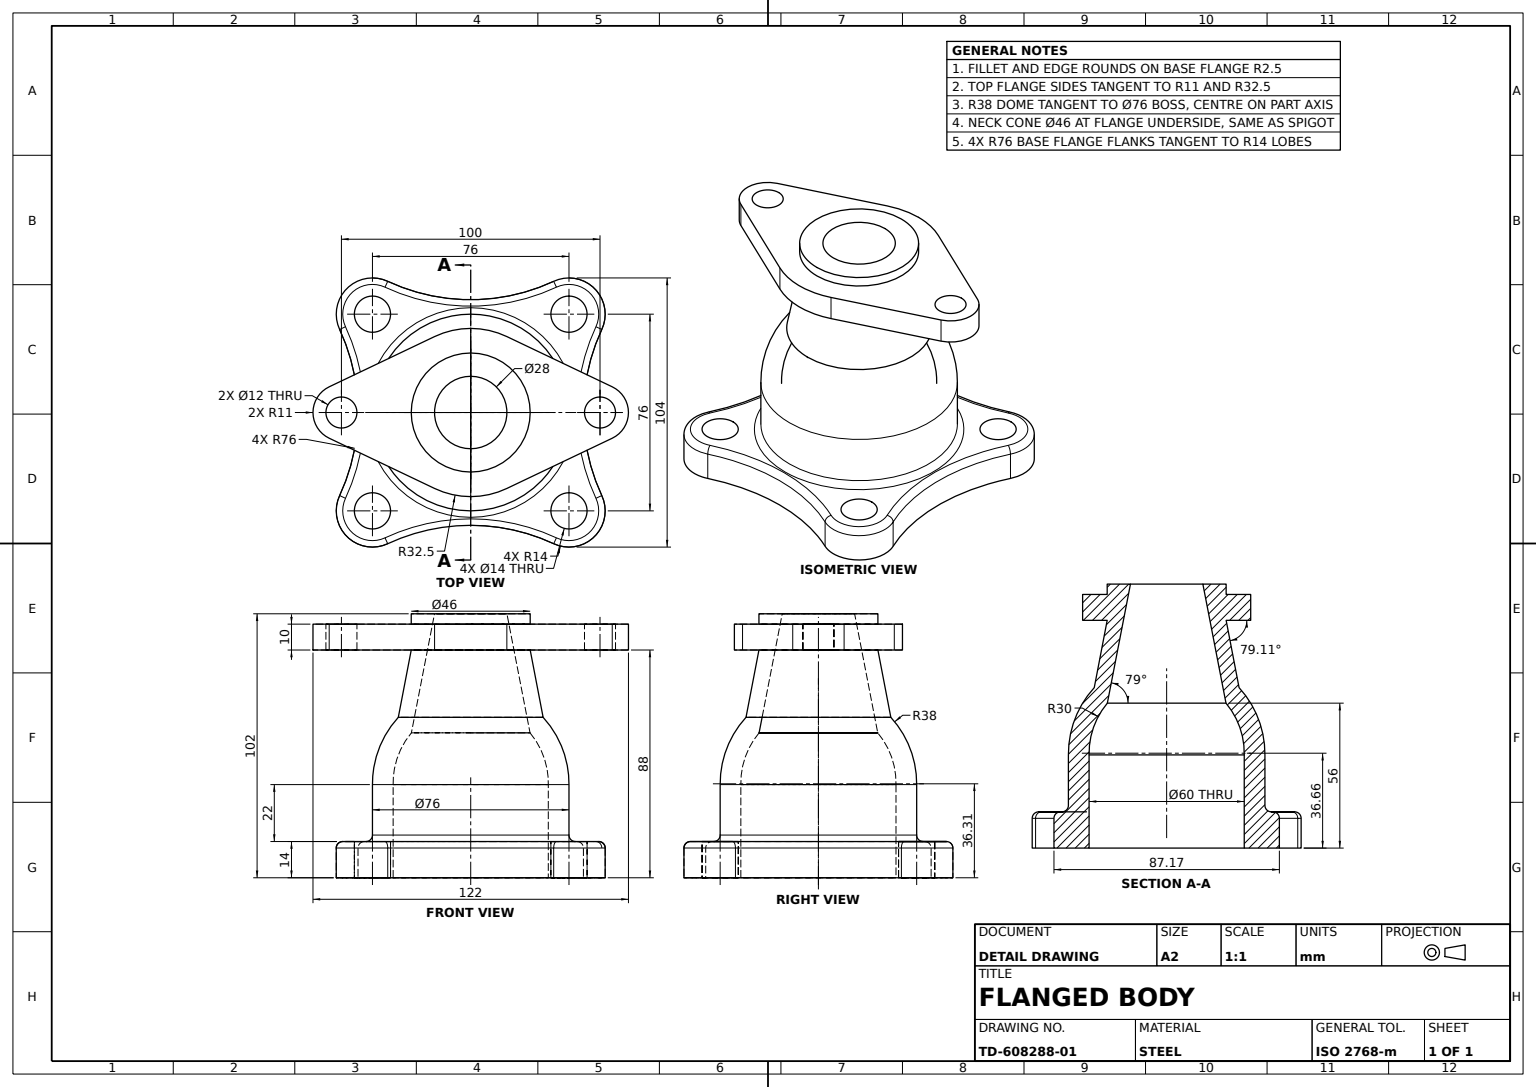
from build123d import *

# Parameters (mm, degrees)
BASE_FLANGE_DEPTH               = 14
BASE_BOSS_SKETCH_R              = 38
BASE_BOSS_76_DEPTH              = 22
NECK_LOFT_UPPER_PROFILE_46_R    = 23
NECK_LOFT_LOWER_PROFILE_R       = 28
TOP_FLANGE_DEPTH                = 10
TOP_SPIGOT_SKETCH_R             = 23
TOP_SPIGOT_46_DEPTH             = 4
BOTTOM_BORE_SKETCH_R            = 30
BOTTOM_BORE_60_DEPTH            = 104.831594421
BASE_MOUNTING_HOLES_SKETCH_R    = 7
BASE_MOUNTING_HOLES_4X_14_DEPTH = 120.033608699
TOP_FLANGE_HOLES_2X_12_REACH    = 128.606
TOP_FLANGE_HOLES_SKETCH_R       = 6
BASE_BOSS_FILLET_R2_5_R         = 2.5


with BuildPart() as part:
    # Base Flange Sketch → Base Flange (new body)
    with BuildSketch(Plane(origin=(0, 0, 0), x_dir=(1, 0, 0), z_dir=(0, 1, 0))):
        with BuildLine():
            ThreePointArc((-32.088888889, 50.690893012), (-47.899494937, 47.899494937), (-50.690893012, 32.088888889))
            ThreePointArc((-50.690893012, 32.088888889), (-43.584312217, 0), (-50.690893012, -32.088888889))
            ThreePointArc((-50.690893012, -32.088888889), (-47.899494937, -47.899494937), (-32.088888889, -50.690893012))
            ThreePointArc((-32.088888889, -50.690893012), (0, -43.584312217), (32.088888889, -50.690893012))
            ThreePointArc((32.088888889, -50.690893012), (47.899494937, -47.899494937), (50.690893012, -32.088888889))
            ThreePointArc((50.690893012, -32.088888889), (43.584312217, 0), (50.690893012, 32.088888889))
            ThreePointArc((50.690893012, 32.088888889), (47.899494937, 47.899494937), (32.088888889, 50.690893012))
            ThreePointArc((32.088888889, 50.690893012), (0, 43.584312217), (-32.088888889, 50.690893012))
        make_face()
    extrude(amount=BASE_FLANGE_DEPTH)

    # Base Boss Sketch → Base Boss Ø76 (add)
    with BuildSketch(Plane(origin=(0, 14, 0), x_dir=(1, 0, 0), z_dir=(0, 1, 0))):
        with Locations(Location((0, 0, 0), (0, 0, 270))):
            Circle(BASE_BOSS_SKETCH_R)
    extrude(amount=BASE_BOSS_76_DEPTH)

    # Ball Body Profile → Ball Body (revolve)
    with BuildSketch(Plane(origin=(0, 0, 0), x_dir=(0, 0, -1), z_dir=(1, 0, 0)), mode=Mode.PRIVATE) as ball_body_sk:
        with BuildLine():
            Line((0, 62), (-28, 62))
            ThreePointArc((-28, 62), (-35.468382669, 49.94937795), (-38, 36))
            Line((-38, 36), (0, 36))
            Line((0, 36), (0, 62))
        make_face()
    revolve(ball_body_sk.sketch.rotate(Axis((0, 14, 0), (0, 1, 0)), 180), axis=Axis((0, 14, 0), (0, 1, 0)))

    # Neck Loft Upper Profile Ø46 → Neck Loft section 0
    with BuildSketch(Plane(origin=(0, 88, 0), x_dir=(1, 0, 0), z_dir=(0, 1, 0))):
        Circle(NECK_LOFT_UPPER_PROFILE_46_R)
    # Neck Loft Lower Profile → Neck Loft section 1
    with BuildSketch(Plane(origin=(0, 62, 0), x_dir=(1, 0, 0), z_dir=(0, 1, 0))):
        Circle(NECK_LOFT_LOWER_PROFILE_R)
    loft()

    # Top Flange Sketch → Top Flange (add)
    with BuildSketch(Plane(origin=(0, 88, 0), x_dir=(1, 0, 0), z_dir=(0, 1, 0))):
        with BuildLine():
            Line((-54.73, 9.931117762), (-13.975, 29.341938842))
            ThreePointArc((-13.975, 29.341938842), (0, 32.5), (13.975, 29.341938842))
            Line((13.975, 29.341938842), (54.73, 9.931117762))
            ThreePointArc((54.73, 9.931117762), (61, 0), (54.73, -9.931117762))
            Line((54.73, -9.931117762), (13.975, -29.341938842))
            ThreePointArc((13.975, -29.341938842), (0, -32.5), (-13.975, -29.341938842))
            Line((-13.975, -29.341938842), (-54.73, -9.931117762))
            ThreePointArc((-54.73, -9.931117762), (-61, 0), (-54.73, 9.931117762))
        make_face()
    extrude(amount=TOP_FLANGE_DEPTH)

    # Top Spigot Sketch → Top Spigot Ø46 (add)
    with BuildSketch(Plane(origin=(0, 98, 0), x_dir=(1, 0, 0), z_dir=(0, 1, 0))):
        with Locations(Location((0, 0, 0), (0, 0, 270))):
            Circle(TOP_SPIGOT_SKETCH_R)
    extrude(amount=TOP_SPIGOT_46_DEPTH)

    # Ball Groove Profile → Ball Groove (revolve, cut)
    with BuildSketch(Plane.XY, mode=Mode.PRIVATE) as ball_groove_sk:
        Polygon((0, 102), (14, 102), (22.94149422, 56), (0, 56), align=None)
    revolve(ball_groove_sk.sketch.rotate(Axis((0, 102, 0), (0, -1, 0)), 90), axis=Axis((0, 102, 0), (0, -1, 0)), mode=Mode.SUBTRACT)

    # Inner Cavity Profile → Inner Cavity (revolve, cut)
    with BuildSketch(Plane.XY, mode=Mode.PRIVATE) as inner_cavity_sk:
        with BuildLine():
            Line((0, 36), (30, 36))
            ThreePointArc((30, 36), (28.297120073, 46.644573206), (22.94149422, 56))
            Line((22.94149422, 56), (0, 56))
            Line((0, 56), (0, 36))
        make_face()
    revolve(inner_cavity_sk.sketch.rotate(Axis((0, 56, 0), (0, -1, 0)), 90), axis=Axis((0, 56, 0), (0, -1, 0)), mode=Mode.SUBTRACT)

    # Bottom Bore Sketch → Bottom Bore Ø60 (cut, through all)
    with BuildSketch(Plane(origin=(0, 36, 0), x_dir=(1, 0, 0), z_dir=(0, 1, 0))):
        with Locations(Location((0, 0, 0), (0, 0, 270))):
            Circle(BOTTOM_BORE_SKETCH_R)
    extrude(amount=-BOTTOM_BORE_60_DEPTH, mode=Mode.SUBTRACT)

    # Base Mounting Holes Sketch → Base Mounting Holes 4xØ14 (cut, through all)
    with BuildSketch(Plane(origin=(0, 14, 0), x_dir=(1, 0, 0), z_dir=(0, 1, 0))):
        with Locations(Location((38, 38, 0), (0, 0, 270))):
            Circle(BASE_MOUNTING_HOLES_SKETCH_R)
        with Locations(Location((38, -38, 0), (0, 0, 270))):
            Circle(BASE_MOUNTING_HOLES_SKETCH_R)
        with Locations(Location((-38, 38, 0), (0, 0, 270))):
            Circle(BASE_MOUNTING_HOLES_SKETCH_R)
        with Locations(Location((-38, -38, 0), (0, 0, 270))):
            Circle(BASE_MOUNTING_HOLES_SKETCH_R)
    extrude(amount=-BASE_MOUNTING_HOLES_4X_14_DEPTH, mode=Mode.SUBTRACT)

    # Top Flange Holes Sketch → Top Flange Holes 2xØ12 (cut, up to next)
    with BuildSketch(Plane(origin=(0, 98, 0), x_dir=(1, 0, 0), z_dir=(0, 1, 0)), mode=Mode.PRIVATE) as top_flange_holes_2x_12_sk1:
        with Locations(Location((50, 0, 0), (0, 0, 270))):
            Circle(TOP_FLANGE_HOLES_SKETCH_R)
    top_flange_holes_2x_12_tool1 = extrude(top_flange_holes_2x_12_sk1.sketch, amount=-TOP_FLANGE_HOLES_2X_12_REACH, mode=Mode.PRIVATE) & part.part
    # Top Flange Holes Sketch → Top Flange Holes 2xØ12 (cut, up to next)
    with BuildSketch(Plane(origin=(0, 98, 0), x_dir=(1, 0, 0), z_dir=(0, 1, 0)), mode=Mode.PRIVATE) as top_flange_holes_2x_12_sk2:
        with Locations(Location((-50, 0, 0), (0, 0, 270))):
            Circle(TOP_FLANGE_HOLES_SKETCH_R)
    top_flange_holes_2x_12_tool2 = extrude(top_flange_holes_2x_12_sk2.sketch, amount=-TOP_FLANGE_HOLES_2X_12_REACH, mode=Mode.PRIVATE) & part.part
    add(top_flange_holes_2x_12_tool1.solids().sort_by_distance((50, 98, 0))[0], mode=Mode.SUBTRACT)
    add(top_flange_holes_2x_12_tool2.solids().sort_by_distance((-50, 98, 0))[0], mode=Mode.SUBTRACT)

    # Base Boss Fillet R2.5
    base_boss_fillet_r2_5_edges = [part.edges().sort_by_distance(p)[0] for p in [
        (0, 14, 43.584312217),
        (47.899494937, 14, 47.899494937),
        (43.584312217, 14, 0),
        (47.899494937, 14, -47.899494937),
        (0, 14, -38),
        (0, 14, -43.584312217),
        (-47.899494937, 14, -47.899494937),
        (-43.584312217, 14, 0),
        (-47.899494937, 14, 47.899494937),
    ]]
    fillet(base_boss_fillet_r2_5_edges, radius=BASE_BOSS_FILLET_R2_5_R)


solid = part.part
